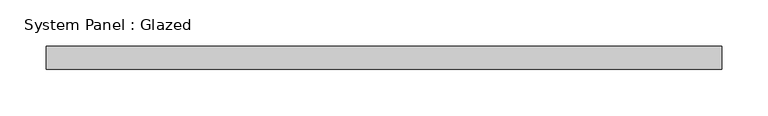
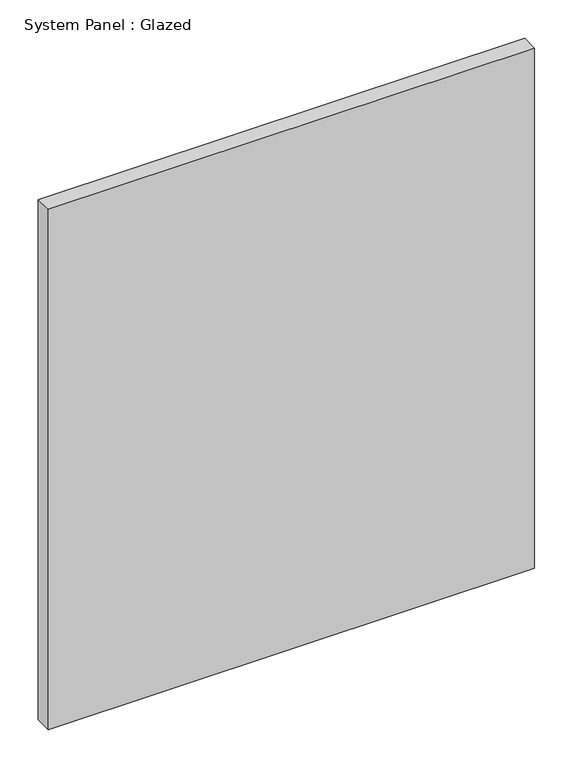
"""IFC4 building model written with IfcOpenShell, lengths in millimetres: plate geometry, System Panel : Glazed."""

from ifc_helpers import new_model, si_unit, origin, origin_with_axes, place, context, project, spatial, polyline, outline, extrude, source, transform, mapped, element, save


def system_panel_glazed_f246ada9(model_context):
    return source(origin(), model_context, "Body", "SweptSolid", [
        extrude(outline(polyline([(365.0, 24.5), (-365.0, 24.5), (-365.0, 49.5), (365.0, 49.5), (365.0, 24.5)])), origin_with_axes(), (0.0, 0.0, 1.0), 825.0),
    ])


if __name__ == "__main__":
    model = new_model("IFC4")
    model_context = context("Model", 3, world=origin())
    ifc_project = project(units=[si_unit("LENGTHUNIT", "METRE", prefix="MILLI")], contexts=[model_context])
    site = spatial("IfcSite", under=ifc_project)
    building = spatial("IfcBuilding", under=site)
    placement = place(None, origin())
    system_panel_glazed_shape = system_panel_glazed_f246ada9(model_context)
    element("IfcPlate", 1, ObjectType="System Panel : Glazed", at=placement, inside=building, context=model_context, shape_type="MappedRepresentation", body=[
        mapped(system_panel_glazed_shape, transform((0.0, 0.0, 0.0), x_axis=(1.0, 0.0, 0.0), y_axis=(0.0, 1.0, 0.0), z_axis=(0.0, 0.0, 1.0))),
    ])
    save(model, "model.ifc")

# Revit data of these elements
# Element 1 (IfcPlate, "System Panel : Glazed")
#   Materials on its faces: "Glass"
# Materials
#   "Glass": class "Glass", colour RGB 218 227 224, transparency 0.85, Description = "Soda Lime Glass", Cost = 0
